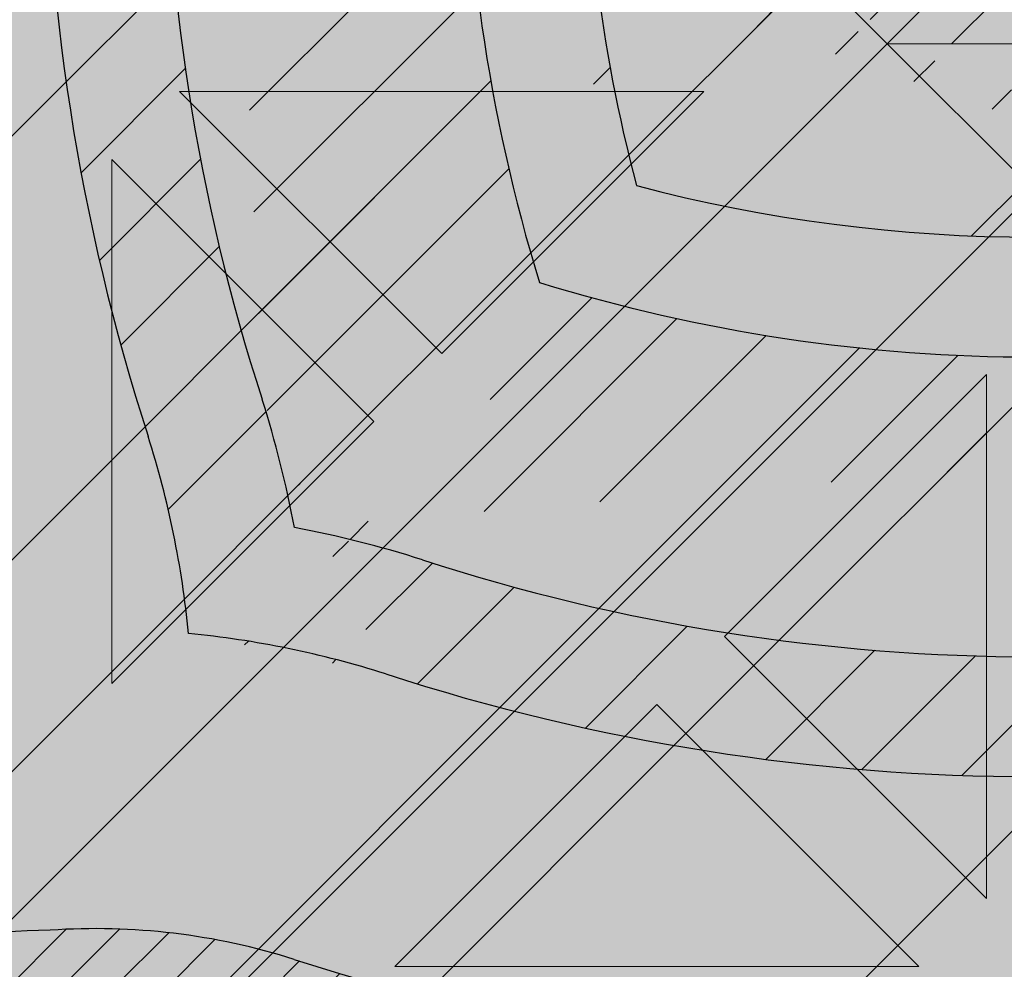
# Model space of a CAD drawing. Units: inches. Extents: x 844 to 2234, y 346 to 1084.
# Tile 54 of 93: x 1866.641 to 1869.26, y 693.802 to 696.327. Entities that reach past the tile are written whole.
import ezdxf

# ---------------------------------------------------------------- set-up
doc = ezdxf.new("R2010")
doc.units = ezdxf.units.IN
doc.header["$MEASUREMENT"] = 0
doc.layers.add('furniture', color=8, linetype='Continuous', lineweight=18)
doc.layers.add('RA-AP-01$0$INT', color=35, linetype='Continuous', lineweight=5)
doc.layers.add('RA-AP-01$0$FURN', color=3, linetype='Continuous')
doc.layers.add('RA-AP-01$0$WOOD', color=64, linetype='Continuous')

# ---------------------------------------------------------------- blocks, each defined once
blk = doc.blocks.new('A$C18D01794')
at = {"layer": 'RA-AP-01$0$INT'}
h = blk.add_hatch(color=256, dxfattribs=at)
h.paths.add_polyline_path([(4.585917135068449, -6.356712009588271), (4.555206456959269, -6.35671200958746), (4.555206456959137, -6.387422687716308), (4.874495778835233, -6.706712009592356), (4.90520645695423, -6.676001331474049)])
h.paths.add_polyline_path([(5.255206456948813, -6.387422687716306), (5.255206456948682, -6.356712009605972), (5.224495778822613, -6.356712009605161), (4.905206456953498, -6.676001331474273), (4.935917135072151, -6.706712009592924)])
h.paths.add_polyline_path([(4.935917135072559, -6.706712009592068), (4.905206456953564, -6.737422687710376), (5.255206456951813, -7.087422687708613), (5.255206456951549, -7.026001331471008)])
h.paths.add_polyline_path([(4.555206456956399, -7.026001331471013), (4.555206456956134, -7.087422687708616), (4.905206456953821, -6.737422687710943), (4.874495778835166, -6.70671200959229)])
h = blk.add_hatch(color=256, dxfattribs=at)
h.paths.add_polyline_path([(4.585917135068448, -6.356712009588273), (4.614201406330596, -6.356712009589021), (4.668846067270487, -6.411356670531338), (4.723490728212344, -6.356712009591912), (4.771774999457151, -6.35671200959319), (4.826419660396886, -6.411356670535356), (4.862780050090322, -6.374996280843536), (4.844495778842715, -6.356712009595112), (4.862780050090411, -6.356712009595595), (4.905206456960182, -6.399138416468211), (4.947632863832445, -6.356712009597838), (4.965917135079675, -6.356712009598322), (4.947632863831759, -6.374996280845421), (4.983993253523576, -6.411356670538857), (5.038637914464627, -6.356712009600247), (5.08692218571208, -6.356712009601523), (5.141566846649976, -6.411356670541852), (5.196211507589851, -6.356712009604411), (5.224495778822615, -6.356712009605161), (4.905206456953975, -6.676001331473793)])
h.paths.add_polyline_path([(4.895206456956031, -6.637717060225675), (4.895206456958921, -6.528427738347902), (4.840561796018589, -6.583072399285802)], flags=16)
h.paths.add_polyline_path([(4.915206456955638, -6.637717060226121), (4.969851117895509, -6.583072399288678), (4.915206456957609, -6.528427738348344)], flags=16)
h.paths.add_polyline_path([(4.826419660395175, -6.568930263661755), (4.881064321335613, -6.514285602723745), (4.771774999456703, -6.514285602720857)], flags=16)
h.paths.add_polyline_path([(4.983993253519558, -6.568930263665262), (5.038637914460456, -6.514285602726792), (4.929348592581548, -6.514285602724816)], flags=16)
h.paths.add_polyline_path([(4.881064321336025, -6.494285602723742), (4.826419660397532, -6.439640941782821), (4.771774999457062, -6.494285602720859)], flags=16)
h.paths.add_polyline_path([(4.929348592582019, -6.494285602724817), (5.038637914460982, -6.494285602726792), (4.983993253522945, -6.439640941786327)], flags=16)
h.paths.add_polyline_path([(4.895206456960191, -6.480143467100443), (4.895206456962115, -6.407422687715913), (4.876922185715016, -6.389138416467584), (4.840561796021581, -6.425498806159401)], flags=16)
h.paths.add_polyline_path([(4.915206456958487, -6.480143467100889), (4.969851117899527, -6.425498806162279), (4.933490728206909, -6.389138416468043), (4.9152064569598, -6.40742268771434)], flags=16)
h.paths.add_polyline_path([(4.757632863832376, -6.480143467096812), (4.812277524772842, -6.425498806158772), (4.757632863834348, -6.370854145217844)], flags=16)
h.paths.add_polyline_path([(4.737632863832376, -6.480143467096286), (4.737632863834348, -6.370854145217375), (4.682988202893906, -6.425498806155385)], flags=16)
h.paths.add_polyline_path([(5.05278005008503, -6.480143467103376), (5.052780050087917, -6.370854145224413), (4.998135389146995, -6.425498806162908)], flags=16)
h.paths.add_polyline_path([(5.072780050085024, -6.480143467103744), (5.127424711025931, -6.42549880616527), (5.072780050087916, -6.370854145224832)], flags=16)
h.paths.add_polyline_path([(4.935917135072783, -6.706712009592292), (5.255206456948811, -6.387422687716309), (5.255206456948932, -6.415706958964177), (5.200561796010279, -6.470351619902839), (5.255206456949403, -6.524996280841948), (5.25520645694961, -6.5732805520894), (5.200561796009787, -6.627925213029239), (5.236922185702417, -6.664285602721864), (5.255206456949919, -6.646001331474357), (5.255206456949998, -6.664285602721898), (5.212780050078687, -6.706712009592262), (5.25520645695036, -6.749138416463932), (5.255206456950438, -6.767422687711313), (5.236922185702424, -6.749138416463297), (5.200561796009796, -6.785498806155928), (5.255206456950753, -6.840143467096874), (5.25520645695096, -6.888427738341682), (5.200561796010322, -6.943072399282328), (5.255206456951428, -6.997717060223427), (5.255206456951547, -7.026001331471006)])
h.paths.add_polyline_path([(5.042988202883395, -6.785498806155427), (5.097632863823085, -6.840143467095101), (5.097632863822622, -6.730854145216193)], flags=16)
h.paths.add_polyline_path([(5.028846067259663, -6.771356670531693), (5.083490728198774, -6.716712009592573), (4.974201406321001, -6.716712009593042)], flags=16)
h.paths.add_polyline_path([(5.117632863823087, -6.840143467095186), (5.172277524762331, -6.785498806155926), (5.11763286382262, -6.730854145216225)], flags=16)
h.paths.add_polyline_path([(5.08349072819877, -6.696712009593886), (5.028846067259652, -6.642067348654775), (4.974201406320998, -6.696712009593438)], flags=16)
h.paths.add_polyline_path([(5.131774999446817, -6.854285602718917), (5.186419660386065, -6.799640941779662), (5.241064321325782, -6.854285602719365)], flags=17)
h.paths.add_polyline_path([(5.131774999446228, -6.716712009592374), (5.186419660386065, -6.771356670532194), (5.222780050079488, -6.734996280838764), (5.204495778832781, -6.716712009592063)], flags=16)
h.paths.add_polyline_path([(5.097632863822613, -6.682569873970264), (5.097632863823061, -6.573280552091354), (5.042988202883383, -6.627925213031044)], flags=16)
h.paths.add_polyline_path([(5.131774999446899, -6.874285602718915), (5.241064321325809, -6.874285602719364), (5.186419660386591, -6.928930263658598)], flags=17)
h.paths.add_polyline_path([(5.131774999446226, -6.696712009594078), (5.204495778830767, -6.696712009594374), (5.22278005007868, -6.67842773834687), (5.186419660386049, -6.642067348654249)], flags=16)
h.paths.add_polyline_path([(5.11763286382262, -6.682569873970225), (5.17227752476232, -6.627925213030515), (5.117632863823064, -6.573280552091267)], flags=16)
h.paths.add_polyline_path([(5.186419660386069, -6.613783077405491), (5.241064321325754, -6.559138416465795), (5.131774999446791, -6.559138416466263)], flags=16)
h.paths.add_polyline_path([(5.131774999446872, -6.539138416466263), (5.24106432132578, -6.539138416465794), (5.186419660386554, -6.484493755526573)], flags=16)
h.paths.add_polyline_path([(5.255206456951811, -7.08742268770861), (5.255206456951895, -7.106712009588038), (4.555206456956052, -7.106712009588038), (4.555206456956136, -7.087422687708617), (4.905206456953973, -6.737422687710788)])
h.paths.add_polyline_path([(4.983993253513404, -6.8444937555241), (4.92934859257295, -6.899138416462108), (5.03863791445186, -6.899138416465014)], flags=16)
h.paths.add_polyline_path([(4.969851117889988, -6.83035161990006), (4.915206456952556, -6.775706958960171), (4.915206456949648, -6.884996280837944)], flags=16)
h.paths.add_polyline_path([(4.929348592572535, -6.919138416462105), (4.983993253511019, -6.973783077403037), (5.038637914451496, -6.919138416465012)], flags=16)
h.paths.add_polyline_path([(5.052780050074912, -6.93328055208906), (4.998135389134438, -6.987925213027088), (5.052780050072919, -7.042569873968025)], flags=16)
h.paths.add_polyline_path([(5.07278005007491, -6.933280552089588), (5.072780050072918, -7.042569873968497), (5.127424711013374, -6.987925213030498)], flags=16)
h.paths.add_polyline_path([(4.89520645695295, -6.775706958959721), (4.840561796013067, -6.830351619897157), (4.895206456950961, -6.884996280837494)], flags=16)
h.paths.add_polyline_path([(4.915206456948365, -6.933280552085403), (4.915206456946434, -7.006001331471951), (4.933490728192729, -7.024285602719066), (4.969851117886972, -6.987925213026453)], flags=16)
h.paths.add_polyline_path([(4.881064321327021, -6.899138416461022), (4.82641966038902, -6.84449375552057), (4.771774999448108, -6.899138416459029)], flags=16)
h.paths.add_polyline_path([(4.895206456950073, -6.933280552084951), (4.840561796009022, -6.987925213023558), (4.876922185700835, -7.024285602716997), (4.895206456948749, -7.006001331469487)], flags=16)
h.paths.add_polyline_path([(4.983993253510392, -7.0020673486505), (4.947632863816944, -7.038427738342319), (4.965917135064043, -7.05671200959023), (5.038637914448995, -7.056712009591555)], flags=16)
h.paths.add_polyline_path([(4.881064321326543, -6.91913841646102), (4.771774999447578, -6.919138416459031), (4.826419660385607, -6.973783077399508)], flags=16)
h.paths.add_polyline_path([(4.905206456946447, -7.014285602717636), (4.862780050074785, -7.056712009588352), (4.947632863816685, -7.056712009589775)], flags=16)
h.paths.add_polyline_path([(5.14156684663679, -7.002067348654549), (5.086922185696452, -7.056712009592438), (5.196211507574223, -7.056712009594425)], flags=16)
h.paths.add_polyline_path([(4.8264196603837, -7.002067348646972), (4.771774999442643, -7.056712009585575), (4.8444957788276, -7.056712009587508), (4.862780050075511, -7.038427738340416)], flags=16)
h.paths.add_polyline_path([(4.812277524760289, -6.98792521302292), (4.757632863822258, -6.933280552082447), (4.757632863819352, -7.042569873961408)], flags=16)
h.paths.add_polyline_path([(4.73763286382226, -6.933280552082079), (4.682988202881349, -6.987925213020536), (4.737632863819352, -7.04256987396099)], flags=16)
h.paths.add_polyline_path([(4.723490728195188, -7.056712009584289), (4.668846067257299, -7.002067348643949), (4.614201406317417, -7.056712009581383)], flags=16)
h.paths.add_polyline_path([(4.597632863829262, -6.706712009592262), (4.555206456957951, -6.664285602721896), (4.555206456958029, -6.646001331474357), (4.573490728205535, -6.664285602721864), (4.609851117898167, -6.627925213029238), (4.555206456958338, -6.573280552089402), (4.555206456958546, -6.524996280841952), (4.60985111789767, -6.470351619902839), (4.555206456959015, -6.415706958964177), (4.555206456959138, -6.387422687716309), (4.874495778835167, -6.70671200959229), (4.5552064569564, -7.026001331471015), (4.555206456956523, -6.997717060223433), (4.609851117897629, -6.94307239928233), (4.555206456956988, -6.888427738341681), (4.555206456957198, -6.840143467096881), (4.609851117898153, -6.78549880615593), (4.573490728205528, -6.749138416463297), (4.555206456957507, -6.76742268771132), (4.555206456957585, -6.749138416463933)])
h.paths.add_polyline_path([(4.712780050085332, -6.730854145216195), (4.712780050084863, -6.840143467095105), (4.767424711024555, -6.785498806155427)], flags=16)
h.paths.add_polyline_path([(4.726922185709173, -6.716712009592573), (4.781566846648288, -6.771356670531693), (4.836211507586949, -6.716712009593043)], flags=16)
h.paths.add_polyline_path([(4.692780050085327, -6.730854145216225), (4.638135389145619, -6.785498806155928), (4.692780050084865, -6.840143467095185)], flags=16)
h.paths.add_polyline_path([(4.726922185709182, -6.696712009593886), (4.836211507586949, -6.696712009593436), (4.7815668466483, -6.642067348654773)], flags=16)
h.paths.add_polyline_path([(4.678637914461726, -6.71671200959237), (4.605917135075169, -6.716712009592063), (4.587632863828464, -6.734996280838766), (4.623993253521887, -6.771356670532195)], flags=16)
h.paths.add_polyline_path([(4.712780050085336, -6.68256987397026), (4.767424711024568, -6.627925213031042), (4.71278005008489, -6.573280552091352)], flags=16)
h.paths.add_polyline_path([(4.678637914461726, -6.696712009594076), (4.623993253521899, -6.642067348654247), (4.587632863829271, -6.67842773834687), (4.605917135077185, -6.696712009594376)], flags=16)
h.paths.add_polyline_path([(4.692780050085336, -6.682569873970228), (4.692780050084889, -6.573280552091267), (4.638135389145632, -6.627925213030515)], flags=16)
h.paths.add_polyline_path([(4.623993253521885, -6.799640941779662), (4.678637914461131, -6.854285602718915), (4.56934859258217, -6.854285602719365)], flags=17)
h.paths.add_polyline_path([(4.623993253521901, -6.613783077405509), (4.678637914461158, -6.559138416466263), (4.569348592582195, -6.559138416465795)], flags=16)
h.paths.add_polyline_path([(4.678637914461051, -6.874285602718915), (4.623993253521361, -6.928930263658598), (4.569348592582143, -6.874285602719364)], flags=17)
h.paths.add_polyline_path([(4.678637914461076, -6.539138416466263), (4.623993253521399, -6.484493755526573), (4.569348592582167, -6.539138416465796)], flags=16)
h = blk.add_hatch(color=256, dxfattribs=at)
h.paths.add_polyline_path([(4.969851117891331, -6.583072399286455), (4.915206456952669, -6.63771706022511), (4.915206456952222, -6.528427738347337)])
h.paths.add_polyline_path([(4.895206456953064, -6.637717060225108), (4.840561796014413, -6.583072399286448), (4.895206456953533, -6.528427738347335)])
h.paths.add_polyline_path([(4.826419660390684, -6.568930263662714), (4.771774999451003, -6.514285602723024), (4.881064321329913, -6.514285602723489)])
h.paths.add_polyline_path([(4.881064321329884, -6.494285602723492), (4.771774999450921, -6.494285602723024), (4.82641966039018, -6.439640941783778)])
h.paths.add_polyline_path([(4.895206456953734, -6.48014346709988), (4.840561796013912, -6.425498806160046), (4.876922185707337, -6.389138416466622), (4.895206456954043, -6.40742268771333)])
h.paths.add_polyline_path([(4.862780050082808, -6.374996280843689), (4.826419660390178, -6.411356670536314), (4.771774999450351, -6.356712009596481), (4.844495778835303, -6.356712009596181)])
h.paths.add_polyline_path([(4.812277524766446, -6.425498806160041), (4.757632863827191, -6.480143467099289), (4.757632863826741, -6.370854145220329)])
h.paths.add_polyline_path([(4.737632863827191, -6.480143467099214), (4.682988202887508, -6.425498806159518), (4.737632863826743, -6.370854145220299)])
h.paths.add_polyline_path([(4.668846067263777, -6.41135667053579), (4.614201406325123, -6.356712009597128), (4.723490728202894, -6.356712009596675)])
h.paths.add_polyline_path([(4.905206456953846, -6.399138416467422), (4.862780050082654, -6.356712009596229), (4.947632863824561, -6.356712009595756)])
h.paths.add_polyline_path([(4.915206456952028, -6.480143467099882), (4.91520645695173, -6.407422687715346), (4.933490728199234, -6.389138416467428), (4.96985111789186, -6.425498806160055)])
h.paths.add_polyline_path([(5.038637914454841, -6.494285602723048), (4.929348592575874, -6.494285602723497), (4.983993253515593, -6.439640941783787)])
h.paths.add_polyline_path([(4.983993253515065, -6.568930263662725), (4.929348592575849, -6.514285602723495), (5.038637914454755, -6.514285602723045)])
h.paths.add_polyline_path([(5.052780050079843, -6.480143467099317), (4.998135389140595, -6.425498806160058), (5.052780050080309, -6.370854145220356)])
h.paths.add_polyline_path([(4.983993253516868, -6.411356670536324), (4.947632863824241, -6.374996280843694), (4.965917135071747, -6.356712009596188), (5.038637914456701, -6.356712009596504)])
h.paths.add_polyline_path([(5.127424711019533, -6.425498806159557), (5.072780050079843, -6.480143467099239), (5.07278005008031, -6.370854145220326)])
h.paths.add_polyline_path([(5.141566846643269, -6.411356670535829), (5.086922185704154, -6.356712009596707), (5.196211507581929, -6.356712009597176)])
h = blk.add_hatch(color=256, dxfattribs=at)
h.paths.add_polyline_path([(4.781566846647504, -6.771356670530272), (4.836211507586161, -6.716712009591613), (4.726922185708388, -6.716712009591159)])
h.paths.add_polyline_path([(4.836211507586161, -6.696712009592008), (4.781566846647504, -6.642067348653354), (4.726922185708388, -6.69671200959247)])
h.paths.add_polyline_path([(4.76742471102377, -6.627925213029623), (4.712780050084083, -6.57328055208994), (4.712780050084542, -6.68256987396885)])
h.paths.add_polyline_path([(4.692780050084544, -6.682569873968819), (4.692780050084084, -6.573280552089856), (4.638135389144834, -6.627925213029111)])
h.paths.add_polyline_path([(4.678637914460932, -6.696712009592669), (4.623993253521102, -6.642067348652844), (4.587632863827676, -6.678427738346266), (4.605917135074382, -6.696712009592973)])
h.paths.add_polyline_path([(4.573490728204743, -6.664285602721736), (4.60985111789737, -6.627925213029108), (4.555206456957541, -6.573280552089279), (4.555206456957237, -6.646001331474231)])
h.paths.add_polyline_path([(4.623993253521098, -6.613783077405377), (4.67863791446035, -6.559138416466126), (4.56934859258139, -6.559138416465669)])
h.paths.add_polyline_path([(4.678637914460275, -6.539138416466126), (4.623993253520583, -6.48449375552644), (4.56934859258136, -6.539138416465672)])
h.paths.add_polyline_path([(4.609851117896854, -6.470351619902707), (4.555206456958196, -6.415706958964051), (4.555206456957738, -6.524996280841822)])
h.paths.add_polyline_path([(4.597632863828475, -6.706712009592775), (4.555206456957283, -6.664285602721582), (4.555206456956805, -6.749138416463489)])
h.paths.add_polyline_path([(4.678637914460932, -6.716712009590963), (4.605917135076396, -6.71671200959066), (4.587632863828479, -6.734996280838164), (4.623993253521104, -6.771356670530792)])
h.paths.add_polyline_path([(4.692780050084091, -6.840143467093776), (4.692780050084548, -6.730854145214809), (4.638135389144834, -6.785498806154524)])
h.paths.add_polyline_path([(4.767424711023772, -6.785498806154004), (4.712780050084545, -6.730854145214786), (4.712780050084089, -6.840143467093692)])
h.paths.add_polyline_path([(4.67863791446036, -6.854285602718778), (4.623993253521105, -6.799640941779527), (4.569348592581399, -6.854285602719237)])
h.paths.add_polyline_path([(4.609851117897371, -6.785498806155798), (4.573490728204743, -6.74913841646317), (4.555206456957237, -6.767422687710675), (4.555206456957548, -6.840143467095629)])
h.paths.add_polyline_path([(4.623993253520596, -6.928930263658465), (4.67863791446028, -6.874285602718778), (4.569348592581367, -6.874285602719238)])
h.paths.add_polyline_path([(4.609851117896867, -6.943072399282199), (4.555206456957749, -6.888427738343082), (4.55520645695821, -6.997717060220857)])
h = blk.add_hatch(color=256, dxfattribs=at)
h.paths.add_polyline_path([(4.905206456953579, -6.70671200959253), (4.905206456953751, -6.676001331474523), (4.874495778835229, -6.706712009592358)])
h.paths.add_polyline_path([(4.935917135071924, -6.706712009592703), (4.905206456953583, -6.706712009592529), (4.90520645695341, -6.737422687710532)])
h = blk.add_hatch(color=256, dxfattribs=at)
h.paths.add_polyline_path([(4.905206456953409, -6.737422687710532), (4.90520645695358, -6.706712009592529), (4.874495778835235, -6.706712009592359)])
h.paths.add_polyline_path([(4.935917135071928, -6.706712009592703), (4.905206456953754, -6.676001331474527), (4.905206456953582, -6.706712009592529)])
for p, q in [((4.905206456953975, -6.676001331473793), (4.585917135071132, -6.356712009590955)), ((4.874495778835167, -6.70671200959229), (4.555206456959136, -6.387422687716307)), ((4.771774999456703, -6.514285602720857), (4.881064321335613, -6.514285602723743)), ((4.826419660395171, -6.568930263661755), (4.771774999456703, -6.514285602720857)), ((4.881064321335613, -6.514285602723743), (4.826419660395173, -6.568930263661757)), ((4.895206456958917, -6.528427738347906), (4.840561796018589, -6.583072399285802)), ((4.895206456958921, -6.528427738347904), (4.895206456956031, -6.637717060225675)), ((4.767424711024566, -6.627925213031041), (4.712780050084888, -6.573280552091352)), ((4.712780050084888, -6.573280552091352), (4.712780050085336, -6.682569873970262)), ((4.895206456956031, -6.637717060225675), (4.840561796018589, -6.583072399285802)), ((4.712780050085336, -6.682569873970262), (4.767424711024568, -6.627925213031042)), ((4.726922185709182, -6.696712009593882), (4.781566846648298, -6.642067348654775)), ((4.836211507586951, -6.696712009593436), (4.781566846648298, -6.642067348654775)), ((4.874495778835233, -6.706712009592356), (4.905206456953753, -6.676001331474525)), ((4.72692218570918, -6.696712009593886), (4.836211507586951, -6.696712009593436)), ((4.874495778835167, -6.70671200959229), (4.555206456956399, -7.026001331471013)), ((4.874495778835233, -6.706712009592356), (4.905206456953409, -6.737422687710532)), ((4.874495778835233, -6.706712009592358), (4.935917135071925, -6.706712009592703))]:
    blk.add_line(p, q, dxfattribs=at)
blk = doc.blocks.new('A$C32926AE1')
at = {"layer": 'RA-AP-01$0$FURN'}
h = blk.add_hatch(dxfattribs=at)
h.set_pattern_fill('ANSI31', color=256, scale=0.1, style=0)
h.set_pattern_definition([(45, (0, 0), (-0.0088388347648318, 0.0088388347648318), [])])
edge = h.paths.add_edge_path(flags=16)
edge.add_arc((4.904771284329206, 4.246793130718756), 0.2603971832811541, 75.22398030683196, 104.7760196931204)
edge.add_arc((4.904771284329206, 4.246793130718756), 0.2603971832811541, 75.223980306832, 104.77601969312039, ccw=False)
edge = h.paths.add_edge_path(flags=16)
edge.add_arc((4.904771284329206, 4.067062675376612), 0.2603971832811541, 255.2239803068796, 284.776019693168)
edge.add_arc((4.904771284329206, 4.067062675376612), 0.2603971832811541, 255.22398030687958, 284.77601969316805, ccw=False)
edge = h.paths.add_edge_path(flags=0)
edge.add_arc((4.904771284329206, 4.067062675376612), 0.2603971832811541, 255.2239803068796, 284.776019693168)
edge.add_arc((4.904771284329206, 4.067062675376612), 0.2603971832811541, 255.22398030687958, 284.77601969316805, ccw=False)
edge = h.paths.add_edge_path(flags=0)
edge.add_arc((4.904771284329206, 4.067062675376612), 0.2603971832811541, 255.2239803068796, 284.776019693168)
edge.add_arc((4.904771284329206, 4.067062675376612), 0.2603971832811541, 255.22398030687958, 284.77601969316805, ccw=False)
edge = h.paths.add_edge_path()
edge.add_arc((4.604388392048174, 4.588829985554312), 0.1599999999999918, 342.3781640246255, 354.4317409793762)
edge.add_arc((5.090145208887507, 4.43216705527679), 0.3503971832811637, 162.0091218307731, 180.3186872093483)
edge.add_arc((5.205154176610243, 4.588829985554953), 0.1599999999999917, 185.5682590208461, 197.6218359767349)
edge.add_arc((4.904771284329229, 4.246793130718735), 0.3503971832811761, 72.00912183053516, 107.9908781690354)
edge.add_arc((9.535952835716557, 4.28682295566602), 4.798342501046485, 178.2875002453811, 181.5576802719453)
edge.add_arc((4.719397359771122, 4.43216705527679), 0.3503971832811637, 359.6813127906516, 377.9908781692269)
edge.add_arc((9.535967292294904, 4.286822350292874), 4.778371420254705, 178.2965938931842, 181.5667745797229)
edge.add_arc((4.719397359771122, 4.43216705527679), 0.3303971832811637, 359.6813127906516, 377.9908781692269)
edge.add_arc((0.2735752763637294, 4.286822350292874), 4.7783714202547, 358.4332254202771, 361.7034061068158)
edge.add_arc((5.061434214606998, 4.732549947558029), 0.1600000000000254, 252.3781640250584, 264.4317409792362)
edge.add_arc((4.748108354051257, 4.732549947558012), 0.1600000000000541, 275.5682590208426, 287.6218359759532)
edge.add_arc((4.604388392048115, 4.588829985554317), 0.1800000000000505, 342.3567572500182, 349.3735009646207)
edge.add_arc((5.205154176610254, 4.588829985554976), 0.1800000000000069, 190.6264990356027, 197.6432427513933)
edge.add_arc((5.061434214607106, 4.732549947558013), 0.1800000000000424, 252.3567572496606, 259.3735009644582)
edge.add_arc((4.904771284329208, 4.246793130718737), 0.3303971832811676, 71.99844483668534, 108.0015551637021)
edge.add_arc((4.748108354051414, 4.732549947558045), 0.1800000000000547, 280.6264990355479, 287.6432427495938)
edge.add_arc((5.090145208887514, 4.432167055276789), 0.2803971832811691, 162.8706300666893, 180.816523289902)
edge.add_arc((4.719397359771136, 4.432167055276689), 0.2803971832811534, 359.183476710103, 377.1293699333214)
edge.add_arc((4.904771284329222, 4.246793130718737), 0.2803971832811769, 72.87063006672916, 107.1293699332334)
edge.add_arc((5.090145208887522, 4.432167055276788), 0.2603971832811776, 165.2239803068007, 180.9953123810312)
edge.add_arc((4.719397359771141, 4.432167055276699), 0.2603971832811458, 359.0046876189768, 374.7760196932087)
edge.add_arc((5.090145208887507, 4.43216705527679), 0.3303971832811637, 162.0091218307731, 180.3186872093483)
edge.add_arc((9.53595427642584, 4.285015535491528), 4.728345371032053, 178.265043920078, 181.5679956281801)
edge.add_arc((0.2735882922327999, 4.285015535491582), 4.728345371032045, 358.4320043718193, 361.7349560799204)
edge.add_arc((9.535953591267507, 4.284458026472751), 4.708343996644348, 178.2573054306777, 181.5704995759608)
edge.add_arc((0.273588977391114, 4.284458026472785), 4.708343996644358, 358.4295004240388, 361.7426945693213)
edge.add_arc((0.2735889773911131, 4.029397779622582), 4.708343996644359, 358.2573054306787, 361.5704995759613)
edge.add_arc((9.535953591267518, 4.029397779622618), 4.708343996644359, 178.4295004240391, 181.7426945693223)
edge.add_arc((0.2735882922327901, 4.028840270603786), 4.728345371032054, 358.2650439200796, 361.5679956281808)
edge.add_arc((9.53595427642584, 4.028840270603841), 4.728345371032054, 178.4320043718199, 181.7349560799219)
edge.add_arc((0.2735752763637302, 4.027033455802493), 4.778371420254699, 358.2965938931842, 361.5667745797229)
edge.add_arc((4.719397359771122, 3.881688750818578), 0.3303971832811637, 342.0091218307731, 360.3186872093484)
edge.add_arc((5.090145208887507, 3.881688750818578), 0.3303971832811637, 179.6813127906516, 197.9908781692269)
edge.add_arc((9.535967292294904, 4.027033455802493), 4.778371420254705, 178.433225420277, 181.7034061068158)
edge.add_arc((4.719397359771122, 3.881688750818578), 0.3503971832811637, 342.0091218307731, 360.3186872093484)
edge.add_arc((9.53595283571655, 4.027032850429349), 4.79834250104648, 178.4423197280546, 181.7124997546188)
edge.add_arc((4.719397359771141, 3.881688750818669), 0.2603971832811458, 345.2239803067913, 360.9953123810232)
edge.add_arc((5.090145208887522, 3.88168875081858), 0.2603971832811776, 179.0046876189687, 194.7760196931993)
edge.add_arc((4.904771284329222, 4.067062675376631), 0.2803971832811769, 252.8706300667665, 287.1293699332708)
edge.add_arc((4.719397359771136, 3.881688750818678), 0.2803971832811534, 342.8706300666787, 360.8165232898969)
edge.add_arc((5.090145208887514, 3.881688750818579), 0.2803971832811691, 179.183476710098, 197.1293699333106)
edge.add_arc((4.748108354051414, 3.581305858537323), 0.1800000000000547, 72.3567572504062, 79.37350096445199)
edge.add_arc((4.904771284329208, 4.067062675376631), 0.3303971832811676, 251.9984448362979, 288.0015551633146)
edge.add_arc((5.061434214607106, 3.581305858537355), 0.1800000000000424, 100.6264990355418, 107.6432427503394)
edge.add_arc((5.205154176610254, 3.725025820540392), 0.1800000000000069, 162.3567572486066, 169.3735009643972)
edge.add_arc((4.604388392048115, 3.725025820541051), 0.1800000000000505, 10.62649903537925, 17.64324274998182)
edge.add_arc((4.748108354051257, 3.581305858537356), 0.1600000000000541, 72.37816402404681, 84.43174097915735)
edge.add_arc((4.904771284329229, 4.067062675376632), 0.3503971832811761, 252.0091218309645, 287.9908781694648)
edge.add_arc((5.061434214606998, 3.581305858537339), 0.1600000000000254, 95.56825902076373, 107.6218359749416)
edge.add_arc((5.205154176610243, 3.725025820540414), 0.1599999999999917, 162.3781640232651, 174.4317409791539)
edge.add_arc((5.090145208887507, 3.881688750818578), 0.3503971832811637, 179.6813127906516, 197.9908781692269)
edge.add_arc((4.604388392048174, 3.725025820541056), 0.1599999999999918, 5.568259020623824, 17.62183597537444)
edge.add_arc((0.2735897329420762, 4.28682295566602), 4.798342501046482, 358.4423197280547, 361.7124997546188)
edge.add_arc((0.2735897329420691, 4.027032850429348), 4.798342501046489, 358.2875002453812, 361.5576802719453)
at = {"layer": 'RA-AP-01$0$WOOD'}
h = blk.add_hatch(color=256, dxfattribs=at)
h.dxf.hatch_style = 1
h.paths.add_polyline_path([(5.157430609644524, 4.573483066760929, -0.1009492694046607), (5.155401577623758, 4.593365984175333, -0.1842662638101597), (5.172249623284174, 4.638795604568598, 0.2056608120311276), (5.179560981299304, 4.661316324430096, 0.3614336704623542), (5.134352340494423, 4.706524965234944, 0.2056608120311297), (5.111831620632933, 4.699213607219793, -0.1842662638101113), (5.066402000239693, 4.682365561559342, -0.1055311479399994), (5.045656153913092, 4.68467289944697, 0.1567636581983829), (4.763886414745334, 4.684672899446966, -0.1055311479399895), (4.743140568418733, 4.68236556155934, -0.1842662638100833), (4.6977109480255, 4.69921360721979, 0.2056608120302612), (4.675190228164109, 4.706524965234949, 0.3614336704708441), (4.629981587358889, 4.66131632442871, 0.2056608120245944), (4.637292945374126, 4.638795604567974, -0.1842662638101024), (4.654140991034615, 4.59336598417475, -0.1009492694055169), (4.652111959013835, 4.573483066760181, 0.021410119221476), (4.629748025606143, 4.156712009541676, 0.0214101192214795), (4.652111959013809, 3.739940952323101, -0.1009492694059586), (4.654140991034615, 3.720058034908448, -0.1842662638100975), (4.637292945374126, 3.674628414515226, 0.2056608120245705), (4.629981587358889, 3.652107694654492, 0.3614336704708879), (4.675190228164113, 3.606899053848249, 0.2056608120302384), (4.697710948025501, 3.614210411863408, -0.1842662638100995), (4.743140568418738, 3.63105845752386, -0.1055311479402541), (4.763886414745388, 3.628751119636215, 0.1567636581983776), (5.045656153913137, 3.628751119636244, -0.1055311479397538), (5.066402000239692, 3.631058457523857, -0.1842662638101067), (5.111831620632931, 3.614210411863407, 0.2056608120310924), (5.134352340494417, 3.606899053848256, 0.3614336704624001), (5.179560981299307, 3.652107694653103, 0.2056608120311314), (5.172249623284175, 3.6746284145146, -0.1842662638101402), (5.155401577623758, 3.72005803490786, -0.1009492694051366), (5.15743060964455, 3.739940952322354, 0.0214101192215073), (5.179794543052287, 4.156712009541468, 0.0214101192215252)])
h.paths.add_polyline_path([(4.639748609479751, 4.156712009541513, 0.0213537860821624), (4.661970494867118, 3.741887061152232, -0.094075836301374), (4.664143710413708, 3.7196126951003, -0.1824818158568985), (4.644813765429836, 3.668037719127816, 0.2056608120245319), (4.639939526753007, 3.653023905887301, 0.3614336704710246), (4.676106439397173, 3.616856993242342, 0.2056608120302234), (4.691120252638095, 3.621731231919122, -0.1824818158602558), (4.742695228611606, 3.641061176902986, -0.1029891339458722), (4.766991894714349, 3.638256818950944, 0.156709409989566), (5.042550673941472, 3.638256818950105, -0.102989133958497), (5.066847340047078, 3.641061176902949, -0.1824818158594995), (5.118422316020358, 3.621731231919103, 0.2056608120311416), (5.133436129261316, 3.616856993242346, 0.3614336704621468), (5.169603041905217, 3.653023905886178, 0.2056608120310986), (5.164728803228477, 3.668037719127177, -0.1824818158565612), (5.145398858244737, 3.719612695099578, -0.0940758363009313), (5.147572073791232, 3.741887061151398, 0.0213537860822023), (5.169793959178681, 4.156712009541451, 0.0213537860822226), (5.147572073791203, 4.571536957931898, -0.0940758363005034), (5.145398858244737, 4.59381132398362, -0.1824818158565587), (5.164728803228476, 4.645386299956021, 0.2056608120311045), (5.169603041905216, 4.66040011319702, 0.3614336704621845), (5.133436129261313, 4.696567025840856, 0.2056608120310773), (5.118422316020359, 4.691692787164098, -0.182481815859508), (5.066847340047078, 4.67236284218025, -0.1029891339584606), (5.04255067394148, 4.675167200133092, 0.156709409989566), (4.766991894714357, 4.675167200132257, -0.1029891339458842), (4.742695228611611, 4.672362842180213, -0.1824818158602725), (4.691120252638095, 4.691692787164077, 0.2056608120302152), (4.676106439397174, 4.696567025840858, 0.3614336704710363), (4.639939526753005, 4.660400113195899, 0.2056608120245495), (4.644813765429837, 4.645386299955384, -0.1824818158568934), (4.664143710413708, 4.593811323982902, -0.0940758363009187), (4.661970494867149, 4.571536957931074, 0.021353786082177)], flags=16)
h.paths.add_polyline_path([(5.129794543052235, 4.432167055276933, -0.0141661062790638), (5.130152669293814, 4.156927903047693, -0.0141661062790647), (5.129794543052234, 3.881688750818433, -0.0785247771143638), (5.10979738006795, 3.755143611847103, 0.0945969212073497), (5.105408519571111, 3.717898134952927, 0.1043170707844957), (5.116074640131521, 3.670385395016088, 0.1043170707864965), (5.068561900193738, 3.681051515576561, 0.09459692119553), (5.031316423304057, 3.676662655080835, -0.1580239521427272), (4.778226145355827, 3.676662655080367, 0.0945969211986668), (4.740980668464973, 3.681051515576592, 0.1043170707882822), (4.693467928526415, 3.670385395015844, 0.1043170707867916), (4.704134049087309, 3.717898134953662, 0.0945969211972894), (4.69974518859162, 3.755143611844042, -0.0785247771163196), (4.679748025606343, 3.881688750818406, -0.0141661062790663), (4.679389899364763, 4.156927903047693, -0.0141661062790672), (4.679748025606343, 4.432167055276998, -0.0785247771163064), (4.699745188591625, 4.55871219425134, 0.094596921197333), (4.704134049087308, 4.595957671141738, 0.1043170707867205), (4.693467928526416, 4.643470411079523, 0.1043170707882628), (4.740980668464965, 4.632804290518776, 0.0945969211988114), (4.778226145355874, 4.637193151015016, -0.158023952142669), (5.031316423304015, 4.637193151014546, 0.0945969211956361), (5.068561900193736, 4.632804290518806, 0.1043170707864979), (5.11607464013152, 4.643470411079278, 0.1043170707844617), (5.105408519571112, 4.595957671142455, 0.0945969212074597), (5.109797380067959, 4.558712194248236, -0.0785247771143467)], flags=0)
h.paths.add_polyline_path([(5.119794532311105, 4.432259799204851, -0.0142000800617244), (5.120156169157484, 4.156927903047701, -0.0142000800617277), (5.119794532311105, 3.881596006890482, -0.0784894509520253), (5.100273383573699, 3.758192358677797, 0.0940138827242913), (5.095413455884425, 3.717477693979438, 0.0606271852308753), (5.099615656341024, 3.686844378806616, 0.0606271852322524), (5.068982341167493, 3.691046579263239, 0.0940138827010453), (5.028267676478798, 3.686186651576848, -0.1580706864508061), (4.781274892180912, 3.686186651576435, 0.0940138827026903), (4.740560227491556, 3.691046579263279, 0.0606271852339895), (4.709926912317155, 3.686844378806508, 0.0606271852329405), (4.714129112773991, 3.717477693980356, 0.094013882701304), (4.709269185087677, 3.758192358669163, -0.0784894509577193), (4.689748036347473, 3.881596006890469, -0.014200080061729), (4.689386399501094, 4.156927903047709, -0.0142000800617217), (4.689748036347473, 4.432259799204808, -0.078489450957724), (4.709269185087651, 4.555663447426125, 0.0940138827014585), (4.714129112773992, 4.596378112114996, 0.0606271852329731), (4.709926912317154, 4.62701142728886, 0.0606271852340196), (4.74056022749157, 4.622809226832087, 0.0940138827024997), (4.781274892180847, 4.627669154518912, -0.1580706864508359), (5.028267676478777, 4.627669154518526, 0.0940138827010946), (5.068982341167492, 4.622809226832129, 0.060627185232254), (5.099615656341024, 4.627011427288751, 0.0606271852308727), (5.095413455884425, 4.59637811211593, 0.0940138827241088), (5.100273383573675, 4.555663447417647, -0.0784894509520978)], flags=0)
h.paths.add_polyline_path([(5.06978912287499, 4.430218106756144, -0.014241683694547), (5.070173729147532, 4.156927903047672, -0.0142416836945458), (5.06978912287499, 3.883637699339223, -0.0800609523125196), (5.052662118612511, 3.773463122773442, 0.0526421978001116), (5.04590916754064, 3.740550867606997, 0.0526421977992423), (5.012996912374707, 3.73379791653534, -0.1583028414718258), (4.796545656286308, 3.73379791653451, 0.0526421978034211), (4.763633401117837, 3.740550867607021, 0.0526421978018622), (4.756880450045755, 3.773463122774558, -0.0800609523117106), (4.739753445783639, 3.883637699339268, -0.0142416836945435), (4.739368839511098, 4.156927903047671, -0.0142416836945477), (4.739753445783639, 4.430218106756155, -0.0800609523116345), (4.75688045004574, 4.540392683320762, 0.052642197801941), (4.763633401117837, 4.573304938488346, 0.0526421978035071), (4.796545656286361, 4.580057889560873, -0.1583028414717561), (5.012996912374669, 4.580057889560039, 0.0526421977993048), (5.04590916754064, 4.57330493848837, 0.0526421978002057), (5.052662118612529, 4.540392683321868, -0.080060952312477)], flags=0)
h.paths.add_polyline_path([(5.049789715110557, 4.43038092723357, -0.0143097550741839), (5.05018085590259, 4.156927903047715, -0.0143097550741854), (5.049789715110558, 3.883474878861827, -0.0800685599149176), (5.03362098255317, 3.779581877367999, 0.0306258898956367), (5.028241146483733, 3.758218888663947, 0.0306258898977031), (5.006878157778253, 3.75283905259408, -0.1583983521624096), (4.802664410878162, 3.752839052594731, 0.0306258898946014), (4.781301422174808, 3.758218888663924, 0.0306258898967912), (4.775921586105202, 3.779581877368794, -0.080068559914251), (4.759752853548071, 3.883474878861786, -0.0143097550741854), (4.759361712756037, 4.156927903047671, -0.0143097550741854), (4.759752853548071, 4.430380927233557, -0.0800685599142479), (4.775921586105193, 4.534273928726546, 0.0306258898968306), (4.781301422174808, 4.555636917431444, 0.0306258898945754), (4.802664410878143, 4.561016753500631, -0.1583983521624168), (5.006878157778244, 4.561016753501291, 0.0306258898977177), (5.028241146483733, 4.555636917431421, 0.0306258898958182), (5.03362098255321, 4.534273928727244, -0.080068559914796)], flags=0)
h.paths.add_polyline_path([(4.999766070382627, 4.428171244713864, -0.0143443147609634), (5.000198441819402, 4.156927903047689, -0.0143443147609612), (4.999766070382627, 3.885684561381556, -0.0784641635803329), (4.987356730658798, 3.799103304488872, -0.1506053783831347), (4.822185837999821, 3.79910330448882, -0.0784641635803318), (4.809776498276007, 3.885684561381509, -0.014344314760963), (4.809344126839227, 4.156927903047677, -0.0143443147609645), (4.809776498276007, 4.428171244713873, -0.0784641635803192), (4.822185837999822, 4.514752501606549, -0.1506053783831338), (4.987356730658798, 4.514752501606494, -0.078464163580285)], flags=0)
h.paths.add_polyline_path([(4.979755254238824, 4.42764379880488, -0.0143772539198268), (4.980205517789977, 4.156927903047693, -0.0143772539198275), (4.979755254238824, 3.886212007290489, -0.0689242507424422), (4.971183264704897, 3.815276770442801, -0.1296645318904179), (4.838359303953726, 3.815276770442746, -0.0689242507424186), (4.829787314419809, 3.886212007290419, -0.0143772539198292), (4.829337050868653, 4.156927903047653, -0.0143772539198325), (4.829787314419809, 4.427643798804946, -0.0689242507424211), (4.838359303953725, 4.498579035652621, -0.1296645318904187), (4.971183264704897, 4.498579035652565, -0.0689242507424401)], flags=0)
h = blk.add_hatch(color=256, dxfattribs=at)
h.dxf.hatch_style = 1
h.paths.add_polyline_path([(5.145398858244737, 4.59381132398362, -0.1824818158565616), (5.164728803228476, 4.645386299956021, 0.2056608120311045), (5.169603041905216, 4.66040011319702, 0.3614336704621845), (5.133436129261313, 4.696567025840856, 0.2056608120310773), (5.118422316020359, 4.691692787164098, -0.182481815859508), (5.066847340047078, 4.67236284218025, -0.1029891339584606), (5.04255067394148, 4.675167200133092, 0.156709409989566), (4.766991894714357, 4.675167200132257, -0.1029891339458842), (4.742695228611611, 4.672362842180213, -0.1824818158602725), (4.691120252638095, 4.691692787164077, 0.2056608120302152), (4.676106439397174, 4.696567025840858, 0.3614336704710363), (4.639939526753005, 4.660400113195899, 0.2056608120245495), (4.644813765429837, 4.645386299955384, -0.1824818158568934), (4.664143710413708, 4.593811323982902, -0.0940758363009187), (4.661970494867149, 4.571536957931074, 0.0213537860821772), (4.639748609479751, 4.156712009541507, 0.0213537860821625), (4.661970494867119, 3.741887061152226, -0.0940758363013071), (4.664143710413708, 3.719612695100309, -0.1824818158569294), (4.644813765429836, 3.668037719127816, 0.2056608120245319), (4.639939526753007, 3.653023905887301, 0.3614336704710246), (4.676106439397173, 3.616856993242342, 0.2056608120302234), (4.691120252638095, 3.621731231919122, -0.1824818158602558), (4.742695228611606, 3.641061176902986, -0.1029891339458722), (4.766991894714349, 3.638256818950944, 0.156709409989566), (5.042550673941472, 3.638256818950105, -0.102989133958497), (5.066847340047078, 3.641061176902949, -0.1824818158594995), (5.118422316020358, 3.621731231919103, 0.2056608120311416), (5.133436129261316, 3.616856993242346, 0.3614336704621468), (5.169603041905217, 3.653023905886178, 0.2056608120310986), (5.164728803228477, 3.668037719127177, -0.1824818158565612), (5.145398858244737, 3.719612695099578, -0.0940758363009313), (5.147572073791232, 3.741887061151398, 0.0213537860822023), (5.169793959178681, 4.156712009541451, 0.0213537860822226), (5.147572073791203, 4.571536957931898, -0.0940758363004996)])
h.paths.add_polyline_path([(5.109797380067958, 4.55871219424824, -0.0785247771143472), (5.129794543052234, 4.432167055276936, -0.0141661062790644), (5.130152669293814, 4.156927903047685, -0.014166106279066), (5.129794543052234, 3.881688750818401, -0.0785247771143517), (5.109797380067946, 3.755143611847092, 0.0945969212073132), (5.105408519571111, 3.717898134952929, 0.1043170707844995), (5.116074640131521, 3.670385395016088, 0.1043170707864965), (5.068561900193738, 3.681051515576561, 0.09459692119553), (5.031316423304057, 3.676662655080835, -0.1580239521427272), (4.778226145355827, 3.676662655080367, 0.0945969211986668), (4.740980668464973, 3.681051515576592, 0.1043170707882822), (4.693467928526415, 3.670385395015844, 0.1043170707867916), (4.704134049087309, 3.717898134953662, 0.0945969211972894), (4.69974518859162, 3.755143611844042, -0.0785247771163196), (4.679748025606343, 3.881688750818406, -0.0141661062790663), (4.679389899364763, 4.156927903047693, -0.0141661062790672), (4.679748025606343, 4.432167055276998, -0.0785247771163064), (4.699745188591625, 4.55871219425134, 0.094596921197333), (4.704134049087308, 4.595957671141738, 0.1043170707867205), (4.693467928526416, 4.643470411079523, 0.1043170707882628), (4.740980668464965, 4.632804290518776, 0.0945969211988114), (4.778226145355874, 4.637193151015016, -0.158023952142669), (5.031316423304015, 4.637193151014546, 0.0945969211956361), (5.068561900193736, 4.632804290518806, 0.1043170707864979), (5.11607464013152, 4.643470411079278, 0.1043170707844617), (5.105408519571112, 4.595957671142455, 0.0945969212074504)], flags=16)
h.paths.add_polyline_path([(5.100273383573655, 4.55566344741771, -0.0784894509521388), (5.119794532311105, 4.432259799204852, -0.0142000800617252), (5.120156169157484, 4.156927903047686, -0.014200080061726), (5.119794532311105, 3.881596006890502, -0.0784894509520446), (5.100273383573696, 3.758192358677786, 0.0940138827242721), (5.095413455884425, 3.717477693979436, 0.0606271852308692), (5.099615656341024, 3.686844378806616, 0.0606271852322522), (5.068982341167493, 3.691046579263239, 0.0940138827010453), (5.028267676478798, 3.686186651576848, -0.1580706864508061), (4.781274892180912, 3.686186651576435, 0.0940138827026903), (4.740560227491556, 3.691046579263279, 0.0606271852339895), (4.709926912317155, 3.686844378806508, 0.0606271852329405), (4.714129112773991, 3.717477693980356, 0.094013882701304), (4.709269185087677, 3.758192358669163, -0.0784894509577193), (4.689748036347473, 3.881596006890469, -0.014200080061729), (4.689386399501094, 4.156927903047709, -0.0142000800617217), (4.689748036347473, 4.432259799204808, -0.078489450957724), (4.709269185087651, 4.555663447426125, 0.0940138827014585), (4.714129112773992, 4.596378112114996, 0.0606271852329731), (4.709926912317154, 4.62701142728886, 0.0606271852340196), (4.74056022749157, 4.622809226832087, 0.0940138827024997), (4.781274892180847, 4.627669154518912, -0.1580706864508359), (5.028267676478777, 4.627669154518526, 0.0940138827010946), (5.068982341167492, 4.622809226832129, 0.060627185232254), (5.099615656341024, 4.627011427288751, 0.0606271852308727), (5.095413455884425, 4.59637811211593, 0.094013882723957)], flags=0)
h.paths.add_polyline_path([(5.04590916754064, 4.57330493848837, 0.0526421978002057), (5.052662118612529, 4.540392683321868, -0.0800609523124783), (5.06978912287499, 4.430218106756142, -0.0142416836945469), (5.070173729147532, 4.156927903047672, -0.0142416836945458), (5.06978912287499, 3.883637699339223, -0.0800609523125196), (5.052662118612511, 3.773463122773442, 0.0526421978001116), (5.04590916754064, 3.740550867606997, 0.0526421977992423), (5.012996912374707, 3.73379791653534, -0.1583028414718258), (4.796545656286308, 3.73379791653451, 0.0526421978034211), (4.763633401117837, 3.740550867607021, 0.0526421978018622), (4.756880450045755, 3.773463122774558, -0.0800609523117106), (4.739753445783639, 3.883637699339268, -0.0142416836945435), (4.739368839511098, 4.156927903047671, -0.0142416836945477), (4.739753445783639, 4.430218106756155, -0.0800609523116345), (4.75688045004574, 4.540392683320762, 0.052642197801941), (4.763633401117837, 4.573304938488346, 0.0526421978035071), (4.796545656286361, 4.580057889560873, -0.1583028414717561), (5.012996912374669, 4.580057889560039, 0.0526421977993048)], flags=0)
h.paths.add_polyline_path([(5.028241146483733, 4.555636917431422, 0.0306258898956949), (5.033620982553182, 4.534273928727329, -0.0800685599148649), (5.049789715110557, 4.430380927233569, -0.0143097550741839), (5.05018085590259, 4.156927903047715, -0.0143097550741854), (5.049789715110558, 3.883474878861827, -0.0800685599149176), (5.03362098255317, 3.779581877367999, 0.0306258898956367), (5.028241146483733, 3.758218888663947, 0.0306258898977031), (5.006878157778253, 3.75283905259408, -0.1583983521624096), (4.802664410878162, 3.752839052594731, 0.0306258898946014), (4.781301422174808, 3.758218888663924, 0.0306258898967912), (4.775921586105202, 3.779581877368794, -0.080068559914251), (4.759752853548071, 3.883474878861786, -0.0143097550741854), (4.759361712756037, 4.156927903047671, -0.0143097550741854), (4.759752853548071, 4.430380927233557, -0.0800685599142479), (4.775921586105193, 4.534273928726546, 0.0306258898968306), (4.781301422174808, 4.555636917431444, 0.0306258898945754), (4.802664410878143, 4.561016753500631, -0.1583983521624168), (5.006878157778244, 4.561016753501291, 0.0306258898977174)], flags=0)
h.paths.add_polyline_path([(4.987356730658798, 4.514752501606494, -0.0784641635803018), (4.999766070382627, 4.428171244713845, -0.0143443147609637), (5.000198441819402, 4.156927903047665, -0.0143443147609622), (4.999766070382628, 3.885684561381514, -0.0784641635802952), (4.987356730658797, 3.799103304488872, -0.1506053783831338), (4.822185837999821, 3.799103304488819, -0.0784641635803342), (4.809776498276007, 3.885684561381512, -0.0143443147609628), (4.809344126839227, 4.156927903047676, -0.0143443147609646), (4.809776498276007, 4.428171244713873, -0.0784641635803192), (4.822185837999822, 4.514752501606549, -0.1506053783831338)], flags=0)
h.paths.add_polyline_path([(4.971183264704897, 4.498579035652566, -0.0689242507424384), (4.979755254238824, 4.427643798804883, -0.0143772539198276), (4.980205517789977, 4.15692790304768, -0.0143772539198258), (4.979755254238823, 3.88621200729051, -0.0689242507424628), (4.971183264704897, 3.815276770442801, -0.129664531890417), (4.838359303953726, 3.815276770442746, -0.0689242507424186), (4.829787314419809, 3.886212007290419, -0.0143772539198292), (4.829337050868653, 4.156927903047653, -0.0143772539198325), (4.829787314419809, 4.427643798804946, -0.0689242507424211), (4.838359303953725, 4.498579035652621, -0.1296645318904187)], flags=0)
h = blk.add_hatch(dxfattribs=at)
h.set_pattern_fill('ANSI31', color=256, scale=0.05, style=0)
h.set_pattern_definition([(45, (0, 0), (-0.0044194173824159, 0.0044194173824159), [])])
h.paths.add_polyline_path([(5.130152669293814, 4.156927903047704, 0.0141661062790657), (5.129794543052234, 4.432167055276982, 0.0777827904001433), (5.110168979996553, 4.557559993161921, -0.0976515123401879), (5.105408519571111, 4.595957671142454, -0.1043170707844687), (5.116074640131522, 4.64347041107928), (5.099615656341024, 4.627011427288751, 0.0606271852308727), (5.095413455884425, 4.59637811211593, 0.0940138827241088), (5.100273383573675, 4.555663447417647, -0.0784894509520972), (5.119794532311105, 4.432259799204852, -0.0142000800617252), (5.120156169157484, 4.156927903047686, -0.014200080061726), (5.119794532311105, 3.881596006890502, -0.0784894509520446), (5.100273383573696, 3.758192358677786, 0.0940138827242721), (5.095413455884425, 3.717477693979436, 0.0606271852308692), (5.099615656341024, 3.686844378806616), (5.116074640131519, 3.67038539501609, -0.1043170707844594), (5.105408519571112, 3.717898134952912, -0.0976515123401594), (5.11016897999655, 3.756295812933435, 0.0777827904001654), (5.129794543052234, 3.881688750818409, 0.0141661062790665)])
h.paths.add_polyline_path([(5.030164222210597, 3.676291055149937, -0.0976515123472002), (5.068561900193739, 3.681051515576561, -0.1043170707864927), (5.116074640131521, 3.670385395016088), (5.099615656341024, 3.686844378806616, 0.0606271852322522), (5.068982341167493, 3.691046579263239, 0.0940138827010453), (5.028267676478798, 3.686186651576848, -0.1580706864508061), (4.781274892180912, 3.686186651576435, 0.0940138827026903), (4.740560227491556, 3.691046579263279, 0.0606271852339913), (4.709926912317154, 3.686844378806508), (4.693467928526416, 3.670385395015845, -0.1043170707882796), (4.740980668464973, 3.681051515576592, -0.0976515123427246), (4.779378346446416, 3.676291055150394, 0.156512506893803)])
h.paths.add_polyline_path([(4.689748036347473, 3.881596006890472, -0.014200080061729), (4.689386399501094, 4.156927903047712, -0.0142000800617195), (4.689748036347473, 4.432259799204768, -0.078489450957742), (4.709269185087648, 4.555663447426114, 0.0940138827014821), (4.714129112773992, 4.596378112114995, 0.0606271852329748), (4.709926912317154, 4.62701142728886), (4.693467928526414, 4.643470411079524, -0.1043170707867939), (4.704134049087309, 4.595957671141706, -0.09765151234893), (4.699373588660725, 4.557559993157876, 0.0777827903975372), (4.679748025606343, 4.432167055276987, 0.0141661062790675), (4.679389899364763, 4.156927903047675, 0.0141661062790641), (4.679748025606343, 3.88168875081843, 0.0777827903975637), (4.699373588660724, 3.756295812937497, -0.0976515123490278), (4.704134049087308, 3.717898134953629, -0.1043170707867196), (4.693467928526416, 3.670385395015845), (4.709926912317155, 3.686844378806508, 0.0606271852329413), (4.714129112773991, 3.717477693980357, 0.0940138827013084), (4.709269185087676, 3.758192358669166, -0.0784894509577192)])
h.paths.add_polyline_path([(4.779378346446434, 4.63756475094498, -0.0976515123427943), (4.740980668464964, 4.632804290518776, -0.1043170707882609), (4.693467928526416, 4.643470411079523), (4.709926912317154, 4.62701142728886, 0.0606271852340196), (4.74056022749157, 4.622809226832087, 0.0940138827024997), (4.781274892180847, 4.627669154518912, -0.1580706864508359), (5.028267676478777, 4.627669154518526, 0.0940138827010946), (5.068982341167492, 4.622809226832129, 0.060627185232254), (5.099615656341024, 4.627011427288751), (5.116074640131521, 4.643470411079279, -0.1043170707865022), (5.068561900193735, 4.632804290518806, -0.0976515123475899), (5.030164222210446, 4.637564750945479, 0.1565125068936924)])
h = blk.add_hatch(dxfattribs=at)
h.set_pattern_fill('ANSI32', color=256, scale=0.2, style=0)
h.set_pattern_definition([(45, (0, 0), (-0.0530330085889911, 0.0530330085889911), []), (45, (0.035355339, 0), (-0.0530330085889911, 0.0530330085889911), [])])
h.paths.add_polyline_path([(5.119794532311105, 4.432259799204823, 0.0777015974868765), (5.10065834347252, 4.554469821747928, -0.0968902511992216), (5.095413455884425, 4.596378112115931, -0.060627185230871), (5.099615656341024, 4.627011427288751, -0.060627185232254), (5.068982341167492, 4.622809226832129, -0.0968902512198245), (5.027074050790956, 4.628054114423209, 0.1564657949319105), (4.782468517866163, 4.628054114422785, -0.0968902512152247), (4.740560227491555, 4.622809226832088, -0.0606271852339878), (4.709926912317155, 4.627011427288859, -0.0606271852329413), (4.714129112773991, 4.596378112115011, -0.0968902512205338), (4.708884225182929, 4.554469821738175, 0.0777015974804443), (4.689748036347473, 4.43225979920482, 0.0142000800617215), (4.689386399501094, 4.156927903047726, 0.0142000800617273), (4.689748036347473, 3.88159600689052, 0.077701597480541), (4.708884225182985, 3.759385984357019, -0.096890251220082), (4.714129112773992, 3.717477693980371, -0.0606271852329731), (4.709926912317154, 3.686844378806507, -0.060627185233988), (4.740560227491554, 3.691046579263279, -0.0968902512152569), (4.782468517866175, 3.685801691672578, 0.1564657949319236), (5.027074050790988, 3.685801691672169, -0.0968902512197451), (5.068982341167491, 3.691046579263239, -0.0606271852322557), (5.099615656341024, 3.686844378806616, -0.0606271852308727), (5.095413455884425, 3.717477693979438, -0.0968902511991229), (5.100658343472507, 3.7593859843474, 0.0777015974868745), (5.119794532311105, 3.8815960068905, 0.014200080061726), (5.120156169157484, 4.156927903047685, 0.0142000800617238)])
h.paths.add_polyline_path([(5.070173729147531, 4.156927903047684, -0.0142416836945481), (5.06978912287499, 3.883637699339191, -0.0800609523125107), (5.052662118612505, 3.773463122773424, 0.0526421978000811), (5.04590916754064, 3.740550867606997, 0.0526421977993214), (5.012996912374658, 3.733797916535325, -0.1583028414717916), (4.796545656286304, 3.733797916534512, 0.0526421978034138), (4.763633401117837, 3.740550867607021, 0.0526421978018622), (4.756880450045755, 3.773463122774558, -0.0800609523117106), (4.739753445783639, 3.883637699339268, -0.0142416836945435), (4.739368839511098, 4.156927903047671, -0.0142416836945477), (4.739753445783639, 4.430218106756155, -0.0800609523116345), (4.75688045004574, 4.540392683320762, 0.052642197801941), (4.763633401117837, 4.573304938488346, 0.0526421978035071), (4.796545656286361, 4.580057889560873, -0.1583028414717561), (5.012996912374669, 4.580057889560039, 0.0526421977993048), (5.04590916754064, 4.57330493848837, 0.0526421978002057), (5.052662118612529, 4.540392683321868, -0.0800609523124783), (5.06978912287499, 4.430218106756142, -0.0142416836945463)], flags=16)
h.paths.add_polyline_path([(5.050180855902591, 4.156927903047686, -0.0143097550741856), (5.049789715110558, 3.883474878861795, -0.0800685599148126), (5.033620982553202, 3.7795818773681, 0.0306258898957837), (5.028241146483733, 3.758218888663947, 0.0306258898977031), (5.006878157778253, 3.75283905259408, -0.1583983521624096), (4.802664410878162, 3.752839052594731, 0.0306258898946014), (4.781301422174808, 3.758218888663924, 0.0306258898967912), (4.775921586105202, 3.779581877368794, -0.080068559914251), (4.759752853548071, 3.883474878861786, -0.0143097550741854), (4.759361712756037, 4.156927903047671, -0.0143097550741854), (4.759752853548071, 4.430380927233557, -0.0800685599142479), (4.775921586105193, 4.534273928726546, 0.0306258898968306), (4.781301422174808, 4.555636917431444, 0.0306258898945754), (4.802664410878143, 4.561016753500631, -0.1583983521624168), (5.006878157778244, 4.561016753501291, 0.0306258898977177), (5.028241146483733, 4.555636917431421, 0.0306258898958182), (5.03362098255321, 4.534273928727244, -0.0800685599147973), (5.049789715110557, 4.430380927233568, -0.0143097550741854)], flags=0)
h.paths.add_polyline_path([(5.000198441819402, 4.15692790304769, -0.0143443147609622), (4.999766070382627, 3.885684561381539, -0.0784641635803169), (4.987356730658798, 3.799103304488873, -0.1506053783831347), (4.822185837999821, 3.79910330448882, -0.0784641635803318), (4.809776498276007, 3.885684561381509, -0.014344314760963), (4.809344126839227, 4.156927903047677, -0.0143443147609645), (4.809776498276007, 4.428171244713873, -0.0784641635803192), (4.822185837999822, 4.514752501606549, -0.1506053783831338), (4.987356730658798, 4.514752501606494, -0.0784641635803018), (4.999766070382627, 4.428171244713845, -0.0143443147609624)], flags=0)
h.paths.add_polyline_path([(4.980205517789976, 4.156927903047707, -0.0143772539198295), (4.979755254238824, 3.886212007290466, -0.06892425074242), (4.971183264704897, 3.815276770442801, -0.129664531890417), (4.838359303953726, 3.815276770442746, -0.0689242507424186), (4.829787314419809, 3.886212007290419, -0.0143772539198292), (4.829337050868653, 4.156927903047653, -0.0143772539198325), (4.829787314419809, 4.427643798804946, -0.0689242507424211), (4.838359303953725, 4.498579035652621, -0.1296645318904187), (4.971183264704897, 4.498579035652565, -0.0689242507424418), (4.979755254238824, 4.427643798804878, -0.0143772539198259)], flags=0)
for centre, radius, start, end in [((5.090145208887514, 3.881688750818579), 0.2803971832811691, 179.183476710098, 197.1293699333106), ((5.090145208887522, 3.88168875081858), 0.2603971832811776, 179.0046876189687, 194.7760196931993), ((5.090145208887507, 3.881688750818578), 0.3503971832811637, 179.6813127906516, 197.9908781692269), ((5.090145208887507, 3.881688750818578), 0.3303971832811637, 179.6813127906516, 197.9908781692269), ((4.904771284329206, 4.067062675376612), 0.2603971832811541, 255.2239803068796, 284.776019693168), ((4.904771284329206, 4.067062675376612), 0.2603971832811541, 255.2239803068796, 284.776019693168), ((4.904771284329222, 4.067062675376631), 0.2803971832811769, 252.8706300667665, 287.1293699332708), ((4.604388392048115, 3.725025820541051), 0.1800000000000505, 10.62649903537925, 17.64324274998182), ((4.604388392048174, 3.725025820541056), 0.1599999999999918, 5.568259020623824, 17.62183597537444), ((4.748108354051414, 3.581305858537323), 0.1800000000000547, 72.3567572504062, 79.37350096445199), ((4.904771284329208, 4.067062675376631), 0.3303971832811676, 251.9984448362979, 288.0015551633146), ((4.748108354051257, 3.581305858537356), 0.1600000000000541, 72.37816402404681, 84.43174097915735), ((4.904771284329229, 4.067062675376632), 0.3503971832811761, 252.0091218309645, 287.9908781694648), ((4.748108354051327, 3.581305858537359), 0.1100000000000303, 72.45144083744763, 93.9346900888063), ((4.742507915094622, 3.563091385939261), 0.1279700159630606, 90.8720682532012, 104.749808972944), ((4.904771284329219, 4.067062675376634), 0.4003971832811741, 252.0350753990311, 287.9649246011635)]:
    blk.add_arc(centre, radius, start, end, dxfattribs=at)
blk = doc.blocks.new('A$C5D2F253E')
at = {"layer": 'RA-AP-01$0$FURN', "xscale": -0.7999999999883585, "yscale": 0.7999999999883585, "zscale": 0.8, "rotation": 90}
blk.add_blockref('A$C18D01794', (-5.687757199772477, 4.75791982714071), dxfattribs=at)
at = {"layer": 'RA-AP-01$0$WOOD', "rotation": 270}
blk.add_blockref('A$C32926AE1', (-4.161339601644158, 5.73852594588169), dxfattribs=at)

msp = doc.modelspace()

# ---------------------------------------------------------------- block references
at = {"layer": 'furniture', "xscale": 15.94108302203742, "yscale": 15.94108302203742, "zscale": 15.94108302203742, "rotation": 90}
msp.add_blockref('A$C5D2F253E', (1882.631064852549, 701.4028671565849), dxfattribs=at)

doc.saveas('drawing.dxf')
